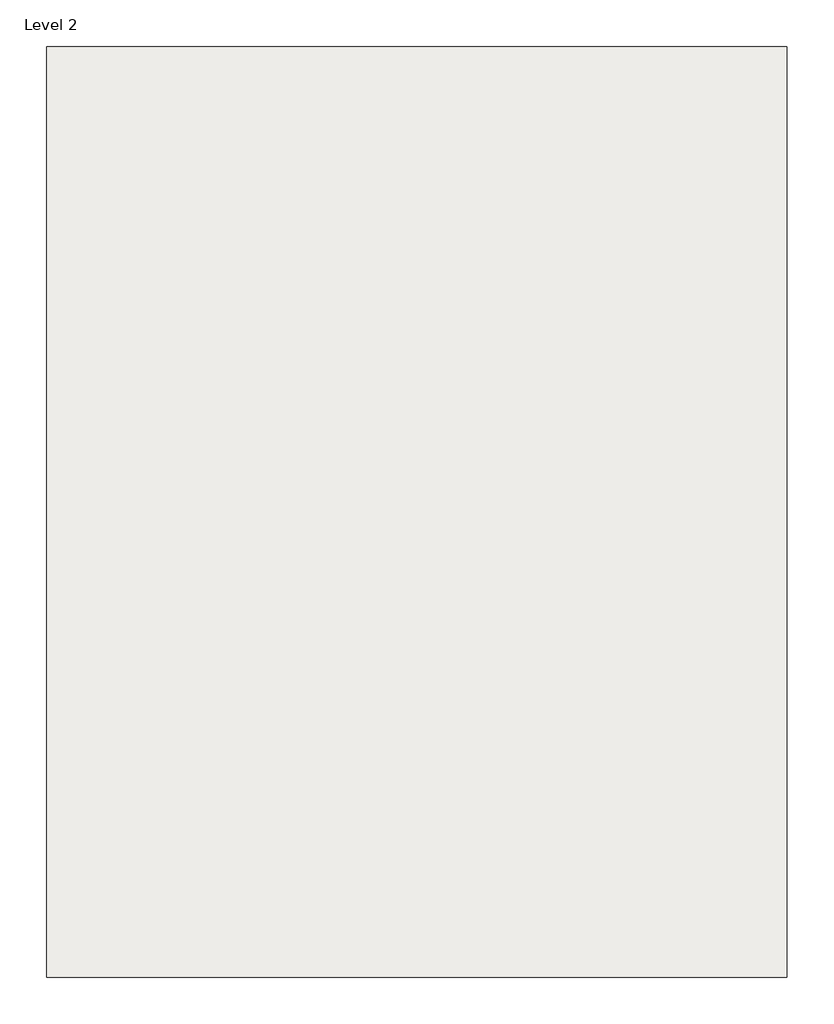
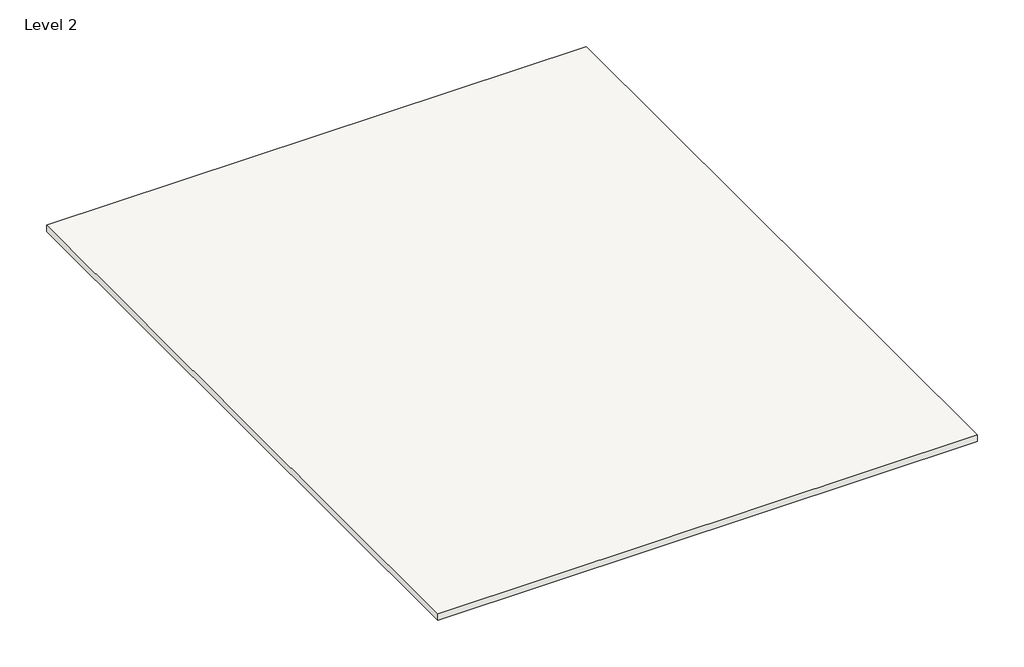
# One storey, incomplete: 1 roof.
"""IFC4 building model written with IfcOpenShell, lengths in millimetres."""

from ifc_helpers import new_model, si_unit, frame, origin, place, context, project, spatial, polyline, outline, extrude, element, save

model = new_model("IFC4")

# Units and contexts
model_context = context("Model", 3, world=origin())
ifc_project = project(units=[si_unit("LENGTHUNIT", "METRE", prefix="MILLI")], contexts=[model_context])

# Site, building, storey
site = spatial("IfcSite", under=ifc_project)
building = spatial("IfcBuilding", under=site)
storey = spatial("IfcBuildingStorey", under=building, Name="Level 2", Elevation=3048.0)

# Roof
placement = place(None, origin())
element("IfcRoof", 1, ObjectType="Generic - 12\"", at=placement, inside=storey, context=model_context, shape_type="SweptSolid", body=[
    extrude(outline(polyline([(-7200.0599931, 8005.7935985), (4687.1400069, 8005.7935985), (4687.1400069, -6929.4064015), (-7200.0599931, -6929.4064015), (-7200.0599931, 8005.7935985)])), frame((0.0, 0.0, 3048.0), z_axis=(0.0, 0.0, 1.0), x_axis=(1.0, 0.0, 0.0)), (0.0, 0.0, 1.0), 152.4),
])

save(model, "model.ifc")

# Revit data of these elements
# Type "Generic - 12\""
#   Assembly Code = "B1020"
#   Layers, outside or top first: 0' - 6" no material (function 1)
# Element 1 (IfcRoof, "Generic - 12\"")
#   built-in parameter 1001705 = 10.5 (stored number, unit not read)
#   built-in parameter 1001710 = 33615
#   Phase Created = New Construction
#   Materials on its faces: "Default Roof", "Oak Flooring"
# Materials
#   "Default Roof": colour RGB 88 101 114, transparency 0, Cost = 0
#   "Oak Flooring": class "Wood", colour RGB 216 169 114, transparency 0, Description = "Quercus Rubra", Cost = 0
